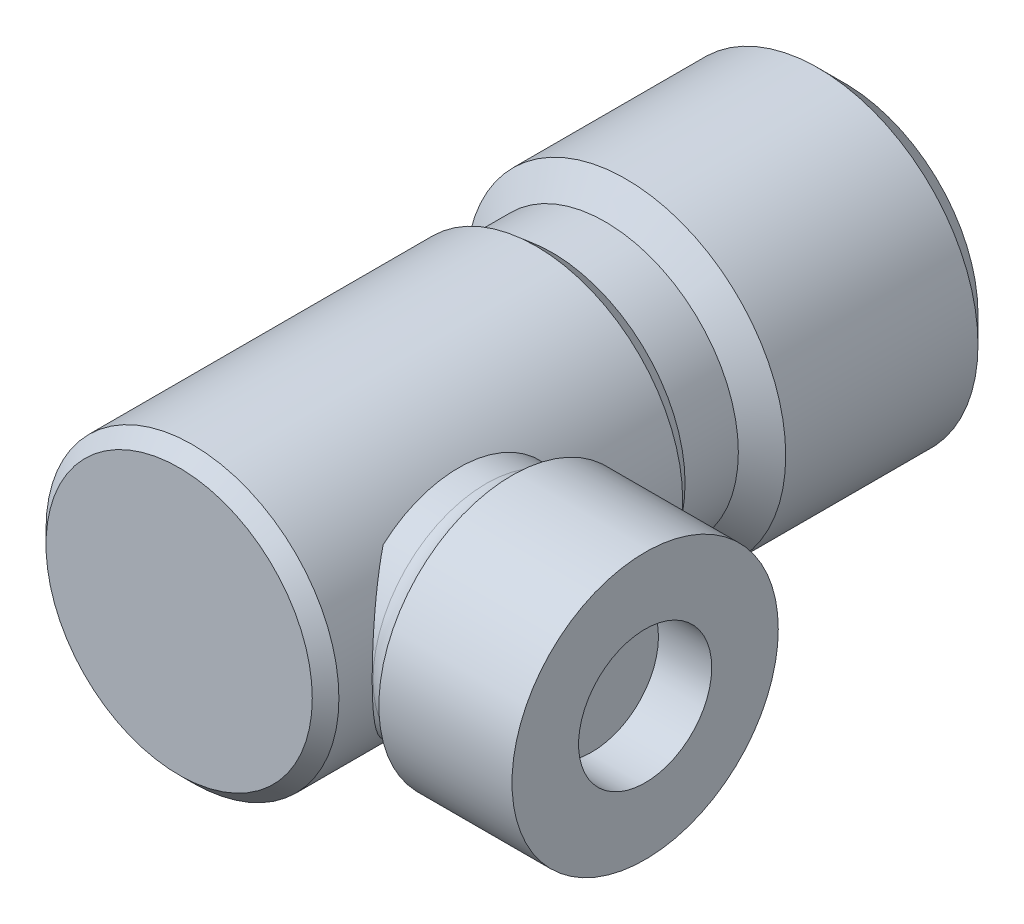
ISO-10303-21;
HEADER;
FILE_DESCRIPTION(('STEP AP214'),'2;1');
FILE_NAME('part.step','',(''),(''),'','','');
FILE_SCHEMA(('AUTOMOTIVE_DESIGN { 1 0 10303 214 1 1 1 1 }'));
ENDSEC;
DATA;
#1=APPLICATION_CONTEXT('core data for automotive mechanical design processes');
#2=APPLICATION_PROTOCOL_DEFINITION('international standard','automotive_design',2000,#1);
#3=PRODUCT_CONTEXT('',#1,'mechanical');
#4=PRODUCT('Part','Part','',(#3));
#5=PRODUCT_RELATED_PRODUCT_CATEGORY('part','',(#4));
#6=PRODUCT_DEFINITION_FORMATION('','',#4);
#7=PRODUCT_DEFINITION_CONTEXT('part definition',#1,'design');
#8=PRODUCT_DEFINITION('design','',#6,#7);
#9=PRODUCT_DEFINITION_SHAPE('','',#8);
#10=(LENGTH_UNIT() NAMED_UNIT(*) SI_UNIT(.MILLI.,.METRE.));
#11=(NAMED_UNIT(*) PLANE_ANGLE_UNIT() SI_UNIT($,.RADIAN.));
#12=(NAMED_UNIT(*) SI_UNIT($,.STERADIAN.) SOLID_ANGLE_UNIT());
#13=UNCERTAINTY_MEASURE_WITH_UNIT(LENGTH_MEASURE(1.E-05),#10,'distance_accuracy_value','');
#14=(GEOMETRIC_REPRESENTATION_CONTEXT(3) GLOBAL_UNCERTAINTY_ASSIGNED_CONTEXT((#13)) GLOBAL_UNIT_ASSIGNED_CONTEXT((#10,
#11,#12)) REPRESENTATION_CONTEXT('',''));
#15=CARTESIAN_POINT('',(0.,0.,0.));
#16=DIRECTION('',(0.,0.,1.));
#17=DIRECTION('',(1.,0.,0.));
#18=AXIS2_PLACEMENT_3D('',#15,#16,#17);
#19=CARTESIAN_POINT('',(0.,0.,0.));
#20=DIRECTION('',(0.,0.,1.));
#21=DIRECTION('',(1.,0.,0.));
#22=AXIS2_PLACEMENT_3D('',#19,#20,#21);
#23=CYLINDRICAL_SURFACE('',#22,5.50000000000001);
#24=CARTESIAN_POINT('',(0.,0.,6.64202465930124));
#25=DIRECTION('',(0.,0.,1.));
#26=DIRECTION('',(1.,0.,0.));
#27=AXIS2_PLACEMENT_3D('',#24,#25,#26);
#28=CIRCLE('',#27,5.50000000000001);
#29=CARTESIAN_POINT('',(5.50000000000001,0.,6.64202465930124));
#30=VERTEX_POINT('',#29);
#31=EDGE_CURVE('E156',#30,#30,#28,.T.);
#32=ORIENTED_EDGE('',*,*,#31,.T.);
#33=EDGE_LOOP('',(#32));
#34=FACE_BOUND('',#33,.T.);
#35=CARTESIAN_POINT('',(0.,0.,19.5506329113924));
#36=DIRECTION('',(0.,0.,1.));
#37=DIRECTION('',(1.,0.,0.));
#38=AXIS2_PLACEMENT_3D('',#35,#36,#37);
#39=CIRCLE('',#38,5.50000000000001);
#40=CARTESIAN_POINT('',(5.50000000000001,0.,19.5506329113924));
#41=VERTEX_POINT('',#40);
#42=EDGE_CURVE('E163',#41,#41,#39,.T.);
#43=ORIENTED_EDGE('',*,*,#42,.F.);
#44=EDGE_LOOP('',(#43));
#45=FACE_BOUND('',#44,.T.);
#46=CARTESIAN_POINT('',(4.5,-3.16227766016839,16.8900870842925));
#47=CARTESIAN_POINT('',(4.55372133798757,-3.08584326423423,16.9751898245627));
#48=CARTESIAN_POINT('',(4.60702109199221,-3.00584312045754,17.0573921441965));
#49=CARTESIAN_POINT('',(4.71183654384651,-2.83871779901779,17.2156730729305));
#50=CARTESIAN_POINT('',(4.76335018130705,-2.75158475850369,17.2917447356478));
#51=CARTESIAN_POINT('',(4.86387500315879,-2.56974361799718,17.4377534798532));
#52=CARTESIAN_POINT('',(4.91286637646493,-2.4749872170038,17.5076444062039));
#53=CARTESIAN_POINT('',(5.00692018041391,-2.27873076407841,17.6400506778738));
#54=CARTESIAN_POINT('',(5.05198437320198,-2.1772337730825,17.7025693356596));
#55=CARTESIAN_POINT('',(5.16600447448915,-1.8968811037625,17.8591287299887));
#56=CARTESIAN_POINT('',(5.23057966474791,-1.71201292790362,17.9459972259891));
#57=CARTESIAN_POINT('',(5.31350857295446,-1.42361098857967,18.0564345413096));
#58=CARTESIAN_POINT('',(5.33881376947333,-1.32571414668223,18.0899162192937));
#59=CARTESIAN_POINT('',(5.38433101520313,-1.1266655041918,18.1498896487857));
#60=CARTESIAN_POINT('',(5.40454562565648,-1.02551536944455,18.1763849157057));
#61=CARTESIAN_POINT('',(5.43956383375897,-0.819827619993593,18.2221521433899));
#62=CARTESIAN_POINT('',(5.45432433516026,-0.715269844583886,18.2413666031624));
#63=CARTESIAN_POINT('',(5.47785022666718,-0.504385580175759,18.2719406276188));
#64=CARTESIAN_POINT('',(5.48661826518229,-0.398059893827932,18.2833036623177));
#65=CARTESIAN_POINT('',(5.49794631016514,-0.184470019740813,18.2979774261312));
#66=CARTESIAN_POINT('',(5.5005032450507,-0.0772053939705694,18.3012841711646));
#67=CARTESIAN_POINT('',(5.49933301058786,0.13722496792917,18.2997697460877));
#68=CARTESIAN_POINT('',(5.49560637469687,0.244390711680658,18.2949492659558));
#69=CARTESIAN_POINT('',(5.48269727460725,0.446246334710113,18.2782202060517));
#70=CARTESIAN_POINT('',(5.47414080392937,0.541044936835875,18.2671246630352));
#71=CARTESIAN_POINT('',(5.45227616927018,0.729156676606386,18.2386987251737));
#72=CARTESIAN_POINT('',(5.43896651122346,0.822469337531874,18.2213663699038));
#73=CARTESIAN_POINT('',(5.39228396443886,1.09915308995716,18.1603691780903));
#74=CARTESIAN_POINT('',(5.35214194670813,1.27949967007459,18.1076844471117));
#75=CARTESIAN_POINT('',(5.25484600104148,1.63458008063911,17.9784543040014));
#76=CARTESIAN_POINT('',(5.19710585861271,1.80884334524746,17.9010814954974));
#77=CARTESIAN_POINT('',(5.06887659876109,2.1420558246331,17.7261657117885));
#78=CARTESIAN_POINT('',(4.99837160852691,2.30098559105912,17.6285976022771));
#79=CARTESIAN_POINT('',(4.85778723728492,2.583332577727,17.4292434291847));
#80=CARTESIAN_POINT('',(4.7887347631536,2.70871064701411,17.3294732652633));
#81=CARTESIAN_POINT('',(4.64671383101553,2.94569556349281,17.1182633678112));
#82=CARTESIAN_POINT('',(4.57376267409195,3.05735700599973,17.006873392813));
#83=CARTESIAN_POINT('',(4.5,3.16227766016839,16.8900870842925));
#84=B_SPLINE_CURVE_WITH_KNOTS('',3,(#46,#47,#48,#49,#50,#51,#52,#53,#54,#55,#56,#57,#58,#59,#60,
#61,#62,#63,#64,#65,#66,#67,#68,#69,#70,#71,#72,#73,#74,#75,#76,#77,#78,#79,#80,#81,#82,#83),
.UNSPECIFIED.,.F.,.F.,(4,2,2,2,2,2,2,2,2,2,2,2,2,2,2,2,2,2,4),(0.,0.379075306582249,
0.75857425876219,1.14070256619167,1.52265851831124,2.16217868668344,2.48140166633247,
2.80046371198673,3.12199552083761,3.4433851344799,3.76493365286404,4.08645487406112,
4.37359627574594,4.66082801390309,5.23460662863761,5.83009545703594,6.42632991315828,
6.94878532198899,7.46908878473004),.UNSPECIFIED.);
#85=CARTESIAN_POINT('',(4.5,-3.16227766016839,16.8900870842925));
#86=VERTEX_POINT('',#85);
#87=CARTESIAN_POINT('',(4.5,3.16227766016839,16.8900870842925));
#88=VERTEX_POINT('',#87);
#89=EDGE_CURVE('E78',#86,#88,#84,.T.);
#90=ORIENTED_EDGE('',*,*,#89,.T.);
#91=DIRECTION('',(0.,0.,1.));
#92=VECTOR('',#91,1.);
#93=CARTESIAN_POINT('',(4.5,3.16227766016839,0.));
#94=LINE('',#93,#92);
#95=CARTESIAN_POINT('',(4.5,3.16227766016839,11.2111787384923));
#96=VERTEX_POINT('',#95);
#97=EDGE_CURVE('E51',#88,#96,#94,.F.);
#98=ORIENTED_EDGE('',*,*,#97,.T.);
#99=CARTESIAN_POINT('',(4.5,3.16227766016839,11.2111787384923));
#100=CARTESIAN_POINT('',(4.55372133798757,3.08584326423423,11.1260759982221));
#101=CARTESIAN_POINT('',(4.60702109199221,3.00584312045754,11.0438736785883));
#102=CARTESIAN_POINT('',(4.71183654384651,2.83871779901779,10.8855927498543));
#103=CARTESIAN_POINT('',(4.76335018130704,2.7515847585037,10.809521087137));
#104=CARTESIAN_POINT('',(4.86387500315879,2.56974361799718,10.6635123429316));
#105=CARTESIAN_POINT('',(4.91286637646493,2.4749872170038,10.5936214165809));
#106=CARTESIAN_POINT('',(5.00692018041391,2.27873076407841,10.461215144911));
#107=CARTESIAN_POINT('',(5.05198437320198,2.1772337730825,10.3986964871252));
#108=CARTESIAN_POINT('',(5.16600447448915,1.8968811037625,10.2421370927961));
#109=CARTESIAN_POINT('',(5.23057966474791,1.71201292790362,10.1552685967957));
#110=CARTESIAN_POINT('',(5.31350857295446,1.42361098857967,10.0448312814752));
#111=CARTESIAN_POINT('',(5.33881376947333,1.32571414668224,10.0113496034911));
#112=CARTESIAN_POINT('',(5.38433101520313,1.1266655041918,9.95137617399908));
#113=CARTESIAN_POINT('',(5.40454562565648,1.02551536944455,9.92488090707913));
#114=CARTESIAN_POINT('',(5.43956383375897,0.819827619993594,9.87911367939489));
#115=CARTESIAN_POINT('',(5.45432433516026,0.715269844583887,9.85989921962243));
#116=CARTESIAN_POINT('',(5.47785022666718,0.50438558017576,9.82932519516597));
#117=CARTESIAN_POINT('',(5.48661826518229,0.398059893827933,9.81796216046712));
#118=CARTESIAN_POINT('',(5.49794631016514,0.184470019740814,9.80328839665365));
#119=CARTESIAN_POINT('',(5.5005032450507,0.0772053939705701,9.79998165162017));
#120=CARTESIAN_POINT('',(5.49933301058786,-0.137224967929169,9.8014960766971));
#121=CARTESIAN_POINT('',(5.49560637469687,-0.244390711680657,9.80631655682901));
#122=CARTESIAN_POINT('',(5.48269727460725,-0.446246334710112,9.82304561673311));
#123=CARTESIAN_POINT('',(5.47414080392937,-0.541044936835875,9.83414115974964));
#124=CARTESIAN_POINT('',(5.45227616927018,-0.729156676606386,9.86256709761107));
#125=CARTESIAN_POINT('',(5.43896651122346,-0.822469337531875,9.87989945288097));
#126=CARTESIAN_POINT('',(5.39228396443886,-1.09915308995716,9.94089664469453));
#127=CARTESIAN_POINT('',(5.35214194670813,-1.27949967007459,9.99358137567313));
#128=CARTESIAN_POINT('',(5.25484600104148,-1.63458008063911,10.1228115187834));
#129=CARTESIAN_POINT('',(5.19710585861271,-1.80884334524746,10.2001843272874));
#130=CARTESIAN_POINT('',(5.06887659876109,-2.1420558246331,10.3751001109964));
#131=CARTESIAN_POINT('',(4.99837160852691,-2.30098559105913,10.4726682205077));
#132=CARTESIAN_POINT('',(4.85778723728492,-2.583332577727,10.6720223936001));
#133=CARTESIAN_POINT('',(4.7887347631536,-2.70871064701411,10.7717925575215));
#134=CARTESIAN_POINT('',(4.64671383101553,-2.94569556349281,10.9830024549736));
#135=CARTESIAN_POINT('',(4.57376267409195,-3.05735700599973,11.0943924299718));
#136=CARTESIAN_POINT('',(4.5,-3.16227766016839,11.2111787384923));
#137=B_SPLINE_CURVE_WITH_KNOTS('',3,(#99,#100,#101,#102,#103,#104,#105,#106,#107,#108,#109,#110,
#111,#112,#113,#114,#115,#116,#117,#118,#119,#120,#121,#122,#123,#124,#125,#126,#127,#128,#129,
#130,#131,#132,#133,#134,#135,#136),.UNSPECIFIED.,.F.,.F.,(4,2,2,2,2,2,2,2,2,2,2,2,2,2,2,2,2,2,
4),(0.,0.379075306582246,0.758574258762189,1.14070256619166,1.52265851831124,2.16217868668344,
2.48140166633247,2.80046371198673,3.12199552083761,3.4433851344799,3.76493365286403,
4.08645487406112,4.37359627574594,4.66082801390309,5.23460662863761,5.83009545703595,
6.42632991315828,6.94878532198899,7.46908878473004),.UNSPECIFIED.);
#138=CARTESIAN_POINT('',(4.5,-3.16227766016839,11.2111787384923));
#139=VERTEX_POINT('',#138);
#140=EDGE_CURVE('E75',#96,#139,#137,.T.);
#141=ORIENTED_EDGE('',*,*,#140,.T.);
#142=DIRECTION('',(0.,0.,1.));
#143=VECTOR('',#142,1.);
#144=CARTESIAN_POINT('',(4.5,-3.16227766016839,0.));
#145=LINE('',#144,#143);
#146=EDGE_CURVE('E82',#139,#86,#145,.T.);
#147=ORIENTED_EDGE('',*,*,#146,.T.);
#148=EDGE_LOOP('',(#90,#98,#141,#147));
#149=FACE_BOUND('',#148,.T.);
#150=ADVANCED_FACE('F43',(#34,#45,#149),#23,.T.);
#151=CARTESIAN_POINT('',(0.,0.,16.3646027128995));
#152=DIRECTION('',(0.,0.,-1.));
#153=DIRECTION('',(-1.,0.,0.));
#154=AXIS2_PLACEMENT_3D('',#151,#152,#153);
#155=CONICAL_SURFACE('',#154,2.5,1.07953834998602);
#156=CARTESIAN_POINT('',(0.,0.,17.7021154812306));
#157=VERTEX_POINT('',#156);
#158=VERTEX_LOOP('',#157);
#159=FACE_BOUND('',#158,.T.);
#160=CARTESIAN_POINT('',(0.,0.,16.3646027128995));
#161=DIRECTION('',(0.,0.,1.));
#162=DIRECTION('',(1.,0.,0.));
#163=AXIS2_PLACEMENT_3D('',#160,#161,#162);
#164=CIRCLE('',#163,2.5);
#165=CARTESIAN_POINT('',(2.5,0.,16.3646027128995));
#166=VERTEX_POINT('',#165);
#167=EDGE_CURVE('E83',#166,#166,#164,.T.);
#168=ORIENTED_EDGE('',*,*,#167,.F.);
#169=EDGE_LOOP('',(#168));
#170=FACE_BOUND('',#169,.T.);
#171=ADVANCED_FACE('F146',(#159,#170),#155,.F.);
#172=CARTESIAN_POINT('',(0.,0.,20.0506329113924));
#173=DIRECTION('',(0.,0.,1.));
#174=DIRECTION('',(1.,0.,0.));
#175=AXIS2_PLACEMENT_3D('',#172,#173,#174);
#176=PLANE('',#175);
#177=CARTESIAN_POINT('',(0.,0.,20.0506329113924));
#178=DIRECTION('',(0.,0.,1.));
#179=DIRECTION('',(1.,0.,0.));
#180=AXIS2_PLACEMENT_3D('',#177,#178,#179);
#181=CIRCLE('',#180,5.00000000000001);
#182=CARTESIAN_POINT('',(5.00000000000001,0.,20.0506329113924));
#183=VERTEX_POINT('',#182);
#184=EDGE_CURVE('E162',#183,#183,#181,.T.);
#185=ORIENTED_EDGE('',*,*,#184,.T.);
#186=EDGE_LOOP('',(#185));
#187=FACE_BOUND('',#186,.T.);
#188=ADVANCED_FACE('F144',(#187),#176,.T.);
#189=CARTESIAN_POINT('',(0.,0.,20.0506329113924));
#190=DIRECTION('',(0.,0.,-1.));
#191=DIRECTION('',(-1.,0.,0.));
#192=AXIS2_PLACEMENT_3D('',#189,#190,#191);
#193=CONICAL_SURFACE('',#192,5.00000000000001,0.785398163397447);
#194=ORIENTED_EDGE('',*,*,#42,.T.);
#195=EDGE_LOOP('',(#194));
#196=FACE_BOUND('',#195,.T.);
#197=ORIENTED_EDGE('',*,*,#184,.F.);
#198=EDGE_LOOP('',(#197));
#199=FACE_BOUND('',#198,.T.);
#200=ADVANCED_FACE('F137',(#196,#199),#193,.T.);
#201=CARTESIAN_POINT('',(0.,0.,6.64202465930124));
#202=DIRECTION('',(0.,0.,1.));
#203=DIRECTION('',(1.,0.,0.));
#204=AXIS2_PLACEMENT_3D('',#201,#202,#203);
#205=CONICAL_SURFACE('',#204,5.50000000000001,0.701854354212814);
#206=CARTESIAN_POINT('',(0.,0.,6.0506329113924));
#207=DIRECTION('',(0.,0.,1.));
#208=DIRECTION('',(1.,0.,0.));
#209=AXIS2_PLACEMENT_3D('',#206,#207,#208);
#210=CIRCLE('',#209,4.99999999999999);
#211=CARTESIAN_POINT('',(4.99999999999999,0.,6.0506329113924));
#212=VERTEX_POINT('',#211);
#213=EDGE_CURVE('E168',#212,#212,#210,.T.);
#214=ORIENTED_EDGE('',*,*,#213,.T.);
#215=EDGE_LOOP('',(#214));
#216=FACE_BOUND('',#215,.T.);
#217=ORIENTED_EDGE('',*,*,#31,.F.);
#218=EDGE_LOOP('',(#217));
#219=FACE_BOUND('',#218,.T.);
#220=ADVANCED_FACE('F138',(#216,#219),#205,.T.);
#221=CARTESIAN_POINT('',(0.,0.,0.));
#222=DIRECTION('',(0.,0.,1.));
#223=DIRECTION('',(1.,0.,0.));
#224=AXIS2_PLACEMENT_3D('',#221,#222,#223);
#225=CYLINDRICAL_SURFACE('',#224,4.99999999999999);
#226=ORIENTED_EDGE('',*,*,#213,.F.);
#227=EDGE_LOOP('',(#226));
#228=FACE_BOUND('',#227,.T.);
#229=CARTESIAN_POINT('',(0.,0.,4.0506329113924));
#230=DIRECTION('',(0.,0.,1.));
#231=DIRECTION('',(1.,0.,0.));
#232=AXIS2_PLACEMENT_3D('',#229,#230,#231);
#233=CIRCLE('',#232,4.99999999999999);
#234=CARTESIAN_POINT('',(4.99999999999999,0.,4.0506329113924));
#235=VERTEX_POINT('',#234);
#236=EDGE_CURVE('E269',#235,#235,#233,.T.);
#237=ORIENTED_EDGE('',*,*,#236,.T.);
#238=EDGE_LOOP('',(#237));
#239=FACE_BOUND('',#238,.T.);
#240=ADVANCED_FACE('F133',(#228,#239),#225,.T.);
#241=CARTESIAN_POINT('',(0.,0.,3.27133112126573));
#242=DIRECTION('',(0.,0.,-1.));
#243=DIRECTION('',(-1.,0.,0.));
#244=AXIS2_PLACEMENT_3D('',#241,#242,#243);
#245=CONICAL_SURFACE('',#244,6.,0.908804282105701);
#246=ORIENTED_EDGE('',*,*,#236,.F.);
#247=EDGE_LOOP('',(#246));
#248=FACE_BOUND('',#247,.T.);
#249=CARTESIAN_POINT('',(0.,0.,3.27133112126573));
#250=DIRECTION('',(0.,0.,1.));
#251=DIRECTION('',(1.,0.,0.));
#252=AXIS2_PLACEMENT_3D('',#249,#250,#251);
#253=CIRCLE('',#252,6.);
#254=CARTESIAN_POINT('',(6.,0.,3.27133112126573));
#255=VERTEX_POINT('',#254);
#256=EDGE_CURVE('E270',#255,#255,#253,.T.);
#257=ORIENTED_EDGE('',*,*,#256,.T.);
#258=EDGE_LOOP('',(#257));
#259=FACE_BOUND('',#258,.T.);
#260=ADVANCED_FACE('F126',(#248,#259),#245,.T.);
#261=CARTESIAN_POINT('',(0.,0.,0.));
#262=DIRECTION('',(0.,0.,1.));
#263=DIRECTION('',(1.,0.,0.));
#264=AXIS2_PLACEMENT_3D('',#261,#262,#263);
#265=CYLINDRICAL_SURFACE('',#264,6.);
#266=ORIENTED_EDGE('',*,*,#256,.F.);
#267=EDGE_LOOP('',(#266));
#268=FACE_BOUND('',#267,.T.);
#269=CARTESIAN_POINT('',(0.,0.,-3.94936708860759));
#270=DIRECTION('',(0.,0.,1.));
#271=DIRECTION('',(1.,0.,0.));
#272=AXIS2_PLACEMENT_3D('',#269,#270,#271);
#273=CIRCLE('',#272,6.);
#274=CARTESIAN_POINT('',(6.,0.,-3.94936708860759));
#275=VERTEX_POINT('',#274);
#276=EDGE_CURVE('E262',#275,#275,#273,.T.);
#277=ORIENTED_EDGE('',*,*,#276,.T.);
#278=EDGE_LOOP('',(#277));
#279=FACE_BOUND('',#278,.T.);
#280=ADVANCED_FACE('F123',(#268,#279),#265,.T.);
#281=CARTESIAN_POINT('',(0.,0.,-4.9493670886076));
#282=DIRECTION('',(0.,0.,1.));
#283=DIRECTION('',(1.,0.,0.));
#284=AXIS2_PLACEMENT_3D('',#281,#282,#283);
#285=CONICAL_SURFACE('',#284,4.99999999999999,0.785398163397448);
#286=ORIENTED_EDGE('',*,*,#276,.F.);
#287=EDGE_LOOP('',(#286));
#288=FACE_BOUND('',#287,.T.);
#289=CARTESIAN_POINT('',(0.,0.,-4.9493670886076));
#290=DIRECTION('',(0.,0.,1.));
#291=DIRECTION('',(1.,0.,0.));
#292=AXIS2_PLACEMENT_3D('',#289,#290,#291);
#293=CIRCLE('',#292,4.99999999999999);
#294=CARTESIAN_POINT('',(4.99999999999999,0.,-4.9493670886076));
#295=VERTEX_POINT('',#294);
#296=EDGE_CURVE('E261',#295,#295,#293,.T.);
#297=ORIENTED_EDGE('',*,*,#296,.T.);
#298=EDGE_LOOP('',(#297));
#299=FACE_BOUND('',#298,.T.);
#300=ADVANCED_FACE('F122',(#288,#299),#285,.T.);
#301=CARTESIAN_POINT('',(0.,0.,-4.9493670886076));
#302=DIRECTION('',(0.,0.,1.));
#303=DIRECTION('',(1.,0.,0.));
#304=AXIS2_PLACEMENT_3D('',#301,#302,#303);
#305=PLANE('',#304);
#306=ORIENTED_EDGE('',*,*,#296,.F.);
#307=EDGE_LOOP('',(#306));
#308=FACE_BOUND('',#307,.T.);
#309=CARTESIAN_POINT('',(0.,0.,-4.9493670886076));
#310=DIRECTION('',(0.,0.,1.));
#311=DIRECTION('',(1.,0.,0.));
#312=AXIS2_PLACEMENT_3D('',#309,#310,#311);
#313=CIRCLE('',#312,4.25);
#314=CARTESIAN_POINT('',(4.25,0.,-4.9493670886076));
#315=VERTEX_POINT('',#314);
#316=EDGE_CURVE('E259',#315,#315,#313,.T.);
#317=ORIENTED_EDGE('',*,*,#316,.T.);
#318=EDGE_LOOP('',(#317));
#319=FACE_BOUND('',#318,.T.);
#320=ADVANCED_FACE('F120',(#308,#319),#305,.F.);
#321=CARTESIAN_POINT('',(0.,0.,-4.9493670886076));
#322=DIRECTION('',(0.,0.,-1.));
#323=DIRECTION('',(-1.,0.,0.));
#324=AXIS2_PLACEMENT_3D('',#321,#322,#323);
#325=CONICAL_SURFACE('',#324,4.25,0.173245666452365);
#326=CARTESIAN_POINT('',(0.,0.,5.0506329113924));
#327=DIRECTION('',(0.,0.,1.));
#328=DIRECTION('',(1.,0.,0.));
#329=AXIS2_PLACEMENT_3D('',#326,#327,#328);
#330=CIRCLE('',#329,2.5);
#331=CARTESIAN_POINT('',(2.5,0.,5.0506329113924));
#332=VERTEX_POINT('',#331);
#333=EDGE_CURVE('E253',#332,#332,#330,.T.);
#334=ORIENTED_EDGE('',*,*,#333,.T.);
#335=EDGE_LOOP('',(#334));
#336=FACE_BOUND('',#335,.T.);
#337=ORIENTED_EDGE('',*,*,#316,.F.);
#338=EDGE_LOOP('',(#337));
#339=FACE_BOUND('',#338,.T.);
#340=ADVANCED_FACE('F113',(#336,#339),#325,.F.);
#341=CARTESIAN_POINT('',(0.,0.,0.));
#342=DIRECTION('',(0.,0.,1.));
#343=DIRECTION('',(1.,0.,0.));
#344=AXIS2_PLACEMENT_3D('',#341,#342,#343);
#345=CYLINDRICAL_SURFACE('',#344,2.5);
#346=ORIENTED_EDGE('',*,*,#167,.T.);
#347=EDGE_LOOP('',(#346));
#348=FACE_BOUND('',#347,.T.);
#349=ORIENTED_EDGE('',*,*,#333,.F.);
#350=EDGE_LOOP('',(#349));
#351=FACE_BOUND('',#350,.T.);
#352=ADVANCED_FACE('F107',(#348,#351),#345,.F.);
#353=CARTESIAN_POINT('',(4.5,0.,14.0506329113924));
#354=DIRECTION('',(1.,0.,0.));
#355=DIRECTION('',(0.,0.,-1.));
#356=AXIS2_PLACEMENT_3D('',#353,#354,#355);
#357=PLANE('',#356);
#358=ORIENTED_EDGE('',*,*,#97,.F.);
#359=CARTESIAN_POINT('',(4.5,0.,14.0506329113924));
#360=DIRECTION('',(1.,0.,0.));
#361=DIRECTION('',(0.,0.,-1.));
#362=AXIS2_PLACEMENT_3D('',#359,#360,#361);
#363=CIRCLE('',#362,4.25);
#364=EDGE_CURVE('E74',#96,#88,#363,.T.);
#365=ORIENTED_EDGE('',*,*,#364,.F.);
#366=EDGE_LOOP('',(#358,#365));
#367=FACE_BOUND('',#366,.T.);
#368=ADVANCED_FACE('F81',(#367),#357,.F.);
#369=CARTESIAN_POINT('',(6.5,0.,14.0506329113924));
#370=DIRECTION('',(-1.,0.,0.));
#371=DIRECTION('',(0.,0.,1.));
#372=AXIS2_PLACEMENT_3D('',#369,#370,#371);
#373=CYLINDRICAL_SURFACE('',#372,4.25);
#374=CARTESIAN_POINT('',(5.53175416344815,0.,14.0506329113924));
#375=DIRECTION('',(1.,0.,0.));
#376=DIRECTION('',(0.,0.,-1.));
#377=AXIS2_PLACEMENT_3D('',#374,#375,#376);
#378=CIRCLE('',#377,4.25);
#379=CARTESIAN_POINT('',(5.53175416344815,0.,9.8006329113924));
#380=VERTEX_POINT('',#379);
#381=EDGE_CURVE('E11',#380,#380,#378,.F.);
#382=ORIENTED_EDGE('',*,*,#381,.T.);
#383=EDGE_LOOP('',(#382));
#384=FACE_BOUND('',#383,.T.);
#385=ORIENTED_EDGE('',*,*,#89,.F.);
#386=EDGE_CURVE('E60',#86,#139,#363,.T.);
#387=ORIENTED_EDGE('',*,*,#386,.T.);
#388=ORIENTED_EDGE('',*,*,#140,.F.);
#389=ORIENTED_EDGE('',*,*,#364,.T.);
#390=EDGE_LOOP('',(#385,#387,#388,#389));
#391=FACE_BOUND('',#390,.T.);
#392=ADVANCED_FACE('F72',(#384,#391),#373,.T.);
#393=ORIENTED_EDGE('',*,*,#146,.F.);
#394=ORIENTED_EDGE('',*,*,#386,.F.);
#395=EDGE_LOOP('',(#393,#394));
#396=FACE_BOUND('',#395,.T.);
#397=ADVANCED_FACE('F106',(#396),#357,.F.);
#398=CARTESIAN_POINT('',(11.5,0.,14.0506329113924));
#399=DIRECTION('',(-1.,0.,0.));
#400=DIRECTION('',(0.,0.,1.));
#401=AXIS2_PLACEMENT_3D('',#398,#399,#400);
#402=CYLINDRICAL_SURFACE('',#401,5.);
#403=CARTESIAN_POINT('',(11.5,0.,14.0506329113924));
#404=DIRECTION('',(1.,0.,0.));
#405=DIRECTION('',(0.,0.,-1.));
#406=AXIS2_PLACEMENT_3D('',#403,#404,#405);
#407=CIRCLE('',#406,5.);
#408=CARTESIAN_POINT('',(11.5,0.,9.0506329113924));
#409=VERTEX_POINT('',#408);
#410=EDGE_CURVE('E246',#409,#409,#407,.T.);
#411=ORIENTED_EDGE('',*,*,#410,.F.);
#412=EDGE_LOOP('',(#411));
#413=FACE_BOUND('',#412,.T.);
#414=CARTESIAN_POINT('',(6.5,0.,14.0506329113924));
#415=DIRECTION('',(1.,0.,0.));
#416=DIRECTION('',(0.,0.,-1.));
#417=AXIS2_PLACEMENT_3D('',#414,#415,#416);
#418=CIRCLE('',#417,5.);
#419=CARTESIAN_POINT('',(6.5,0.,9.0506329113924));
#420=VERTEX_POINT('',#419);
#421=EDGE_CURVE('E245',#420,#420,#418,.T.);
#422=ORIENTED_EDGE('',*,*,#421,.T.);
#423=EDGE_LOOP('',(#422));
#424=FACE_BOUND('',#423,.T.);
#425=ADVANCED_FACE('F167',(#413,#424),#402,.T.);
#426=CARTESIAN_POINT('',(11.5,0.,14.0506329113924));
#427=DIRECTION('',(1.,0.,0.));
#428=DIRECTION('',(0.,0.,-1.));
#429=AXIS2_PLACEMENT_3D('',#426,#427,#428);
#430=PLANE('',#429);
#431=CARTESIAN_POINT('',(11.5,0.,14.0506329113924));
#432=DIRECTION('',(1.,0.,0.));
#433=DIRECTION('',(0.,0.,-1.));
#434=AXIS2_PLACEMENT_3D('',#431,#432,#433);
#435=CIRCLE('',#434,2.5);
#436=CARTESIAN_POINT('',(11.5,0.,11.5506329113924));
#437=VERTEX_POINT('',#436);
#438=EDGE_CURVE('E243',#437,#437,#435,.T.);
#439=ORIENTED_EDGE('',*,*,#438,.F.);
#440=EDGE_LOOP('',(#439));
#441=FACE_BOUND('',#440,.T.);
#442=ORIENTED_EDGE('',*,*,#410,.T.);
#443=EDGE_LOOP('',(#442));
#444=FACE_BOUND('',#443,.T.);
#445=ADVANCED_FACE('F172',(#441,#444),#430,.T.);
#446=CARTESIAN_POINT('',(5.53175416344815,0.,14.0506329113924));
#447=DIRECTION('',(1.,0.,0.));
#448=DIRECTION('',(0.,0.,-1.));
#449=AXIS2_PLACEMENT_3D('',#446,#447,#448);
#450=TOROIDAL_SURFACE('',#449,5.25,1.);
#451=ORIENTED_EDGE('',*,*,#381,.F.);
#452=EDGE_LOOP('',(#451));
#453=FACE_BOUND('',#452,.T.);
#454=ORIENTED_EDGE('',*,*,#421,.F.);
#455=EDGE_LOOP('',(#454));
#456=FACE_BOUND('',#455,.T.);
#457=ADVANCED_FACE('F44',(#453,#456),#450,.F.);
#458=CARTESIAN_POINT('',(9.5,0.,14.0506329113924));
#459=DIRECTION('',(1.,0.,0.));
#460=DIRECTION('',(0.,0.,-1.));
#461=AXIS2_PLACEMENT_3D('',#458,#459,#460);
#462=CYLINDRICAL_SURFACE('',#461,2.5);
#463=CARTESIAN_POINT('',(9.5,0.,14.0506329113924));
#464=DIRECTION('',(1.,0.,0.));
#465=DIRECTION('',(0.,0.,-1.));
#466=AXIS2_PLACEMENT_3D('',#463,#464,#465);
#467=CIRCLE('',#466,2.5);
#468=CARTESIAN_POINT('',(9.5,0.,11.5506329113924));
#469=VERTEX_POINT('',#468);
#470=EDGE_CURVE('E241',#469,#469,#467,.T.);
#471=ORIENTED_EDGE('',*,*,#470,.F.);
#472=EDGE_LOOP('',(#471));
#473=FACE_BOUND('',#472,.T.);
#474=ORIENTED_EDGE('',*,*,#438,.T.);
#475=EDGE_LOOP('',(#474));
#476=FACE_BOUND('',#475,.T.);
#477=ADVANCED_FACE('F218',(#473,#476),#462,.F.);
#478=CARTESIAN_POINT('',(9.5,0.,14.0506329113924));
#479=DIRECTION('',(1.,0.,0.));
#480=DIRECTION('',(0.,0.,-1.));
#481=AXIS2_PLACEMENT_3D('',#478,#479,#480);
#482=PLANE('',#481);
#483=ORIENTED_EDGE('',*,*,#470,.T.);
#484=EDGE_LOOP('',(#483));
#485=FACE_BOUND('',#484,.T.);
#486=ADVANCED_FACE('F228',(#485),#482,.T.);
#487=CLOSED_SHELL('',(#150,#171,#188,#200,#220,#240,#260,#280,#300,#320,#340,#352,#368,#392,
#397,#425,#445,#457,#477,#486));
#488=MANIFOLD_SOLID_BREP('B2',#487);
#489=ADVANCED_BREP_SHAPE_REPRESENTATION('',(#18,#488),#14);
#490=SHAPE_DEFINITION_REPRESENTATION(#9,#489);
ENDSEC;
END-ISO-10303-21;
